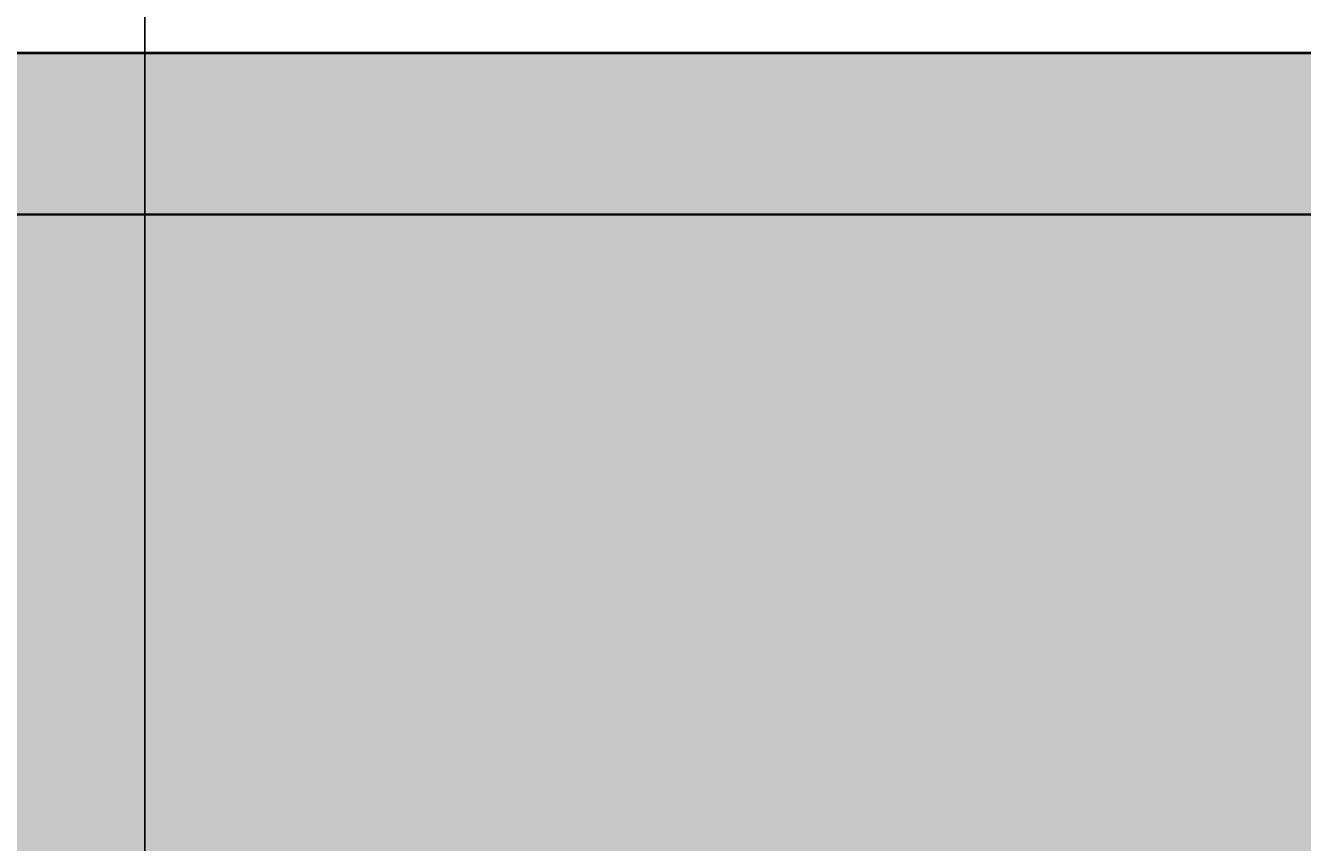
# Model space of a CAD drawing. Units: feet. Extents: x 2695 to 2912, y 795 to 1139.
# Tile 80 of 83: x 2840 to 2876, y 1086 to 1109. Entities that reach past the tile are written whole.
import ezdxf

# ---------------------------------------------------------------- set-up
doc = ezdxf.new("R2010")
doc.units = ezdxf.units.FT
for name, color, linetype, lineweight in [('A-ANNO-DIMS', 2, 'Continuous', 18), ('A-ELEV', 7, 'Continuous', 35), ('A-ELEV-PATT', 252, 'Continuous', 13)]:
    doc.layers.add(name, color=color, linetype=linetype, lineweight=lineweight)
doc.styles.get("Standard").update_dxf_attribs({"font": 'arial.ttf'})
doc.dimstyles.get("Standard").update_dxf_attribs({"dimtxt": 0.18, "dimasz": 0.18, "dimexe": 0.18, "dimexo": 0.0625, "dimgap": 0.09, "dimtad": 0, "dimtih": 1, "dimtoh": 1, "dimdec": 1, "dimzin": 0, "dimdsep": 46, "dimlunit": 3, "dimtxsty": 'Standard', "dimcen": 0.09, "dimadec": 0, "dimazin": 0, "dimtfac": 1, "dimtdec": 1, "dimtofl": 0, "dimtmove": 0, "dimatfit": 3, "dimfxl": 1, "dimtolj": 1, "dimtzin": 0, "dimarcsym": 0})

# ---------------------------------------------------------------- blocks, each defined once
blk = doc.blocks.new('*D10')
at = {"layer": 'A-ANNO-DIMS', "color": 0, "lineweight": -2, "transparency": 16777216}
for p, q in [((2778.034, 1020.886), (2778.034, 1138.886)), ((2778.214, 1138.706), (2810.411, 1138.706)), ((2843.395, 1138.706), (2811.198, 1138.706)), ((2843.575, 1020.886), (2843.575, 1138.886))]:
    blk.add_line(p, q, dxfattribs=at)
at = {"layer": 'A-ANNO-DIMS', "color": 0, "transparency": 16777216}
for points in [[(2778.214, 1138.736), (2778.214, 1138.676), (2778.034, 1138.706)], [(2843.395, 1138.736), (2843.395, 1138.676), (2843.575, 1138.706)]]:
    blk.add_solid(points, dxfattribs=at)
at = {"layer": 'Defpoints', "color": 0, "transparency": 16777216}
for p in [(2843.575, 1138.706), (2778.034, 1020.824), (2843.575, 1020.824)]:
    blk.add_point(p, dxfattribs=at)
at = {"layer": 'A-ANNO-DIMS', "color": 0, "transparency": 16777216, "insert": (2810.805, 1138.706), "char_height": 0.18, "attachment_point": 5}
blk.add_mtext('\\A1;65.54', dxfattribs=at)
blk = doc.blocks.new('*D11')
at = {"layer": 'A-ANNO-DIMS', "color": 0, "lineweight": -2, "transparency": 16777216}
for p, q in [((2843.575, 1020.886), (2843.575, 1138.886)), ((2843.755, 1138.706), (2869.128, 1138.706)), ((2895.289, 1138.706), (2869.916, 1138.706)), ((2895.469, 1107.898), (2895.469, 1138.886))]:
    blk.add_line(p, q, dxfattribs=at)
at = {"layer": 'A-ANNO-DIMS', "color": 0, "transparency": 16777216}
for points in [[(2843.755, 1138.736), (2843.755, 1138.676), (2843.575, 1138.706)], [(2895.289, 1138.736), (2895.289, 1138.676), (2895.469, 1138.706)]]:
    blk.add_solid(points, dxfattribs=at)
at = {"layer": 'Defpoints', "color": 0, "transparency": 16777216}
for p in [(2895.469, 1138.706), (2895.469, 1107.835), (2843.575, 1020.824)]:
    blk.add_point(p, dxfattribs=at)
at = {"layer": 'A-ANNO-DIMS', "color": 0, "transparency": 16777216, "insert": (2869.522, 1138.706), "char_height": 0.18, "attachment_point": 5}
blk.add_mtext('\\A1;51.89', dxfattribs=at)
blk = doc.blocks.new('*D22')
at = {"layer": 'A-ANNO-DIMS', "color": 0, "lineweight": -2, "transparency": 16777216}
for p, q in [((2770.699, 1122.931), (2911.424, 1122.931)), ((2911.244, 1122.751), (2911.244, 1115.565)), ((2911.244, 1108.015), (2911.244, 1115.201)), ((2895.532, 1107.835), (2911.424, 1107.835))]:
    blk.add_line(p, q, dxfattribs=at)
at = {"layer": 'A-ANNO-DIMS', "color": 0, "transparency": 16777216}
for points in [[(2911.214, 1122.751), (2911.274, 1122.751), (2911.244, 1122.931)], [(2911.214, 1108.015), (2911.274, 1108.015), (2911.244, 1107.835)]]:
    blk.add_solid(points, dxfattribs=at)
at = {"layer": 'Defpoints', "color": 0, "transparency": 16777216}
for p in [(2770.636, 1122.931), (2911.244, 1122.931), (2895.469, 1107.835)]:
    blk.add_point(p, dxfattribs=at)
at = {"layer": 'A-ANNO-DIMS', "color": 0, "transparency": 16777216, "insert": (2911.244, 1115.383), "char_height": 0.18, "attachment_point": 5}
blk.add_mtext('\\A1;15.095', dxfattribs=at)
blk = doc.blocks.new('*D50')
at = {"layer": 'A-ANNO-DIMS', "color": 0, "lineweight": -2, "transparency": 16777216}
for p, q in [((2810.041, 972.03), (2810.041, 1138.886)), ((2810.221, 1138.706), (2848.721, 1138.706)), ((2888.008, 1138.706), (2849.508, 1138.706)), ((2888.188, 972.03), (2888.188, 1138.886))]:
    blk.add_line(p, q, dxfattribs=at)
at = {"layer": 'A-ANNO-DIMS', "color": 0, "transparency": 16777216}
for points in [[(2810.221, 1138.736), (2810.221, 1138.676), (2810.041, 1138.706)], [(2888.008, 1138.736), (2888.008, 1138.676), (2888.188, 1138.706)]]:
    blk.add_solid(points, dxfattribs=at)
at = {"layer": 'Defpoints', "color": 0, "transparency": 16777216}
for p in [(2888.188, 1138.706), (2810.041, 971.967), (2888.188, 971.967)]:
    blk.add_point(p, dxfattribs=at)
at = {"layer": 'A-ANNO-DIMS', "color": 0, "transparency": 16777216, "insert": (2849.114, 1138.706), "char_height": 0.18, "attachment_point": 5}
blk.add_mtext('\\A1;78.15', dxfattribs=at)

msp = doc.modelspace()

# ---------------------------------------------------------------- hatches: boundary and pattern name
at = {"layer": 'A-ELEV-PATT'}
h = msp.add_hatch(color=256, dxfattribs=at)
h.set_gradient(color1=(255, 255, 255), tint=1)
h.paths.add_polyline_path([(2770.6361, 1122.9306), (2710.6361, 1122.9306), (2710.6361, 1118.4096), (2770.6361, 1118.4096)])
h.paths.add_polyline_path([(2890.6361, 1107.8588), (2770.6361, 1107.8588), (2770.6361, 1103.3378), (2890.6361, 1103.3378)])
h.paths.add_polyline_path([(2890.6361, 1062.9306), (2710.6361, 1062.9306), (2710.6361, 1056.9306), (2710.6361, 936.9306), (2710.6361, 924.3105), (2716.5358, 924.3105), (2890.6361, 924.3105), (2890.6361, 936.9306), (2715.8852, 936.9306), (2715.8852, 1050.3105), (2890.6361, 1050.3105)])
h.paths.add_polyline_path([(2716.5358, 924.3105), (2710.6361, 924.3105), (2710.6361, 810.9306), (2716.5358, 810.9306)])
h = msp.add_hatch(color=256, dxfattribs=at)
h.set_gradient(color1=(147, 149, 152), color2=(147, 149, 152), tint=1)
h.paths.add_polyline_path([(2770.6361, 1118.4096), (2710.6361, 1118.4096), (2710.6361, 1062.9306), (2770.6361, 1062.9306)])
h.paths.add_polyline_path([(2890.6361, 1103.3378), (2770.6361, 1103.3378), (2770.6361, 1062.9306), (2890.6361, 1062.9306)])
h.paths.add_polyline_path([(2730.7081, 1048.1052), (2755.1125, 1048.1052), (2755.1125, 936.9306), (2770.6361, 936.9306), (2770.6361, 1050.3105), (2715.8852, 1050.3105), (2715.8852, 936.9306), (2730.7081, 936.9306)])
h.paths.add_polyline_path([(2890.6361, 1050.3105), (2770.6361, 1050.3105), (2770.6361, 971.9673), (2778.0341, 971.9673), (2778.0341, 1020.8235), (2843.575, 1020.8235), (2843.575, 971.9673), (2890.6361, 971.9673)])
h.paths.add_polyline_path([(2888.1882, 970.7156), (2843.575, 970.7156), (2843.575, 964.8267), (2888.1882, 964.8267)])
h.paths.add_polyline_path([(2888.1882, 964.1328), (2843.575, 964.1328), (2843.575, 956.614), (2888.1882, 956.614)])
h.paths.add_polyline_path([(2888.1882, 955.9202), (2843.575, 955.9202), (2843.575, 949.2892), (2888.1882, 949.2892)])
h.paths.add_polyline_path([(2888.1882, 948.5954), (2843.575, 948.5954), (2843.575, 941.3507), (2888.1882, 941.3507)])
h.paths.add_polyline_path([(2888.1882, 940.6569), (2843.575, 940.6569), (2843.575, 936.9306), (2888.1882, 936.9306)])
h.paths.add_polyline_path([(2890.6361, 970.7156), (2888.9368, 970.7156), (2888.9368, 964.8267), (2890.6361, 964.8267)])
h.paths.add_polyline_path([(2890.6361, 964.1328), (2888.9368, 964.1328), (2888.9368, 956.614), (2890.6361, 956.614)])
h.paths.add_polyline_path([(2890.6361, 955.9202), (2888.9368, 955.9202), (2888.9368, 949.2892), (2890.6361, 949.2892)])
h.paths.add_polyline_path([(2890.6361, 940.6569), (2888.9368, 940.6569), (2888.9368, 936.9306), (2890.6361, 936.9306)])
h.paths.add_polyline_path([(2890.6361, 948.5954), (2888.9368, 948.5954), (2888.9368, 941.3507), (2890.6361, 941.3507)])
h.paths.add_polyline_path([(2772.5216, 970.7156), (2770.6361, 970.7156), (2770.6361, 964.8267), (2772.5216, 964.8267)])
h.paths.add_polyline_path([(2772.5216, 964.1328), (2770.6361, 964.1328), (2770.6361, 956.614), (2772.5216, 956.614)])
h.paths.add_polyline_path([(2772.5216, 955.9202), (2770.6361, 955.9202), (2770.6361, 949.2892), (2772.5216, 949.2892)])
h.paths.add_polyline_path([(2772.5216, 948.5954), (2770.6361, 948.5954), (2770.6361, 941.3507), (2772.5216, 941.3507)])
h.paths.add_polyline_path([(2772.5216, 940.6569), (2770.6361, 940.6569), (2770.6361, 936.9306), (2772.5216, 936.9306)])
h.paths.add_polyline_path([(2778.0341, 940.6569), (2773.2702, 940.6569), (2773.2702, 936.9306), (2778.0341, 936.9306)])
h.paths.add_polyline_path([(2778.0341, 970.7156), (2773.2702, 970.7156), (2773.2702, 964.8267), (2778.0341, 964.8267)])
h.paths.add_polyline_path([(2778.0341, 964.1328), (2773.2702, 964.1328), (2773.2702, 956.614), (2778.0341, 956.614)])
h.paths.add_polyline_path([(2778.0341, 955.9202), (2773.2702, 955.9202), (2773.2702, 949.2892), (2778.0341, 949.2892)])
h.paths.add_polyline_path([(2778.0341, 948.5954), (2773.2702, 948.5954), (2773.2702, 941.3507), (2778.0341, 941.3507)])
h.paths.add_polyline_path([(2810.0407, 940.6569), (2780.0341, 940.6569), (2780.0341, 936.9306), (2810.0407, 936.9306)])
h.paths.add_polyline_path([(2890.6361, 924.3105), (2770.6361, 924.3105), (2770.6361, 810.9306), (2773.5029, 810.9306), (2773.5029, 905.5143), (2805.9398, 905.5143), (2838.3767, 905.5143), (2838.3767, 810.9306), (2890.6361, 810.9306)])
h = msp.add_hatch(color=256, dxfattribs=at)
h.set_gradient(color1=(199, 200, 202), color2=(213, 227, 240), centered=1)
h.paths.add_polyline_path([(2890.6361, 1103.3378), (2770.6361, 1103.3378), (2770.6361, 1062.9306), (2890.6361, 1062.9306)])

# ---------------------------------------------------------------- linework, layer by layer
at = {"layer": 'A-ELEV'}
for p, q in [((2770.6361, 1107.8588), (2890.6361, 1107.8588)), ((2895.4694, 1107.8352), (2770.6361, 1107.8588)), ((2770.6361, 1103.3378), (2895.4694, 1103.3378))]:
    msp.add_line(p, q, dxfattribs=at)
msp.add_lwpolyline([(2770.6361, 1103.3378), (2890.6361, 1103.3378)], dxfattribs=at)

# ---------------------------------------------------------------- dimensions: what is measured, and where the dimension line sits
at = {"layer": 'A-ANNO-DIMS'}
for base, p1, p2, picture, middle in [((2843.575, 1138.7056), (2778.0341, 1020.8235), (2843.575, 1020.8235), '*D10', (2810.8045, 1138.7056)), ((2888.1882, 1138.7056), (2810.0407, 971.9673), (2888.1882, 971.9673), '*D50', (2849.1144, 1138.7056)), ((2895.4694, 1138.7056), (2843.575, 1020.8235), (2895.4694, 1107.8352), '*D11', (2869.5222, 1138.7056))]:
    dim = msp.add_linear_dim(base=base, p1=p1, p2=p2, dimstyle='Standard', override={"dimdec": 2, "dimlfac": 1, "dimrnd": 0, "dimzin": 0, "dimdsep": 46, "dimlunit": 2}, dxfattribs=at)
    dim.commit()
    dim.dimension.update_dxf_attribs({"geometry": picture, "text_midpoint": middle})
dim = msp.add_linear_dim(base=(2911.2444, 1122.9306), p1=(2895.4694, 1107.8352), p2=(2770.6361, 1122.9306), angle=90, dimstyle='Standard', override={"dimdec": 3, "dimlfac": 1, "dimrnd": 0, "dimzin": 0, "dimdsep": 46, "dimlunit": 2}, dxfattribs=at)
dim.commit()
dim.dimension.update_dxf_attribs({"geometry": '*D22', "text_midpoint": (2911.2444, 1115.3829)})

doc.saveas('drawing.dxf')
